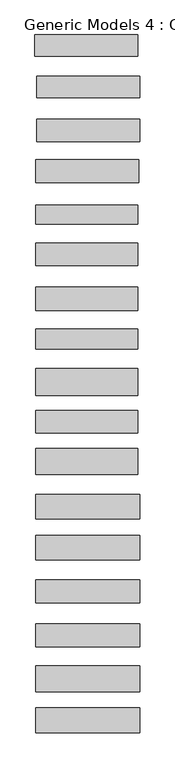
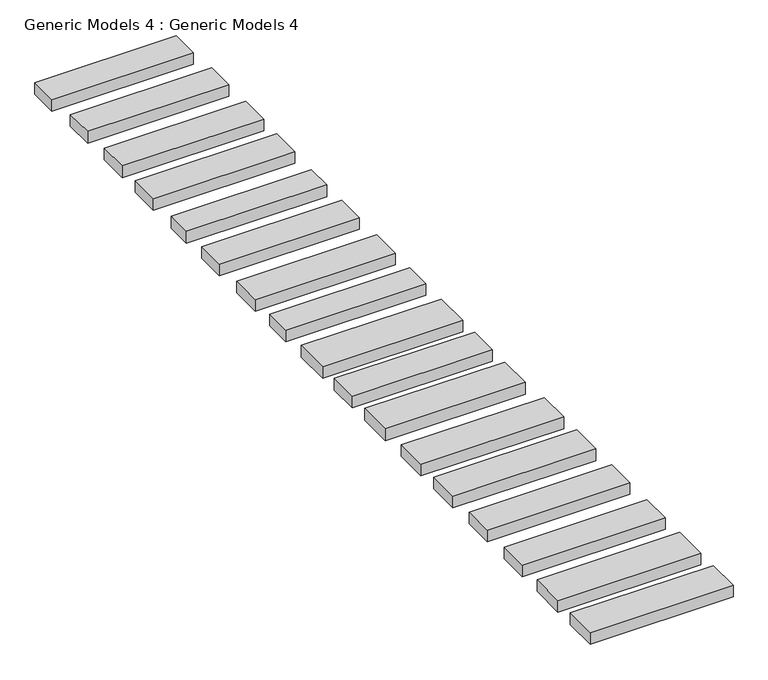
"""IFC4 building model written with IfcOpenShell, lengths in millimetres: proxy geometry, Generic Models 4 : Generic Models 4."""

from ifc_helpers import new_model, si_unit, frame, origin, place, context, project, spatial, polyline, outline, extrude, source, transform, mapped, element, save


def generic_models_4_generic_models_4_6f48c335(model_context):
    return source(origin(), model_context, "Body", "SweptSolid", [
        extrude(outline(polyline([(-33990.9791975, 27174.9938465), (-33990.9791975, 27102.9548339), (-34336.8215134, 27102.9548339), (-34336.8215134, 27174.9938465), (-33990.9791975, 27174.9938465)])), frame((0.0, 0.0, 449.9570313), z_axis=(0.0, 0.0, 1.0), x_axis=(1.0, 0.0, 0.0)), (0.0, 0.0, 1.0), 30.0632812),
        extrude(outline(polyline([(-33984.6291975, 27035.2938465), (-33984.6291975, 26963.2548339), (-34330.4715134, 26963.2548339), (-34330.4715134, 27035.2938465), (-33984.6291975, 27035.2938465)])), frame((0.0, 0.0, 449.9570313), z_axis=(0.0, 0.0, 1.0), x_axis=(1.0, 0.0, 0.0)), (0.0, 0.0, 1.0), 30.0632812),
        extrude(outline(polyline([(-33984.6291975, 26891.4711637), (-33984.6291975, 26815.9588418), (-34330.4715134, 26815.9588418), (-34330.4715134, 26891.4711637), (-33984.6291975, 26891.4711637)])), frame((0.0, 0.0, 449.9570313), z_axis=(0.0, 0.0, 1.0), x_axis=(1.0, 0.0, 0.0)), (0.0, 0.0, 1.0), 30.0632812),
        extrude(outline(polyline([(-33987.8041975, 26754.691992), (-33987.8041975, 26678.491992), (-34333.6465134, 26678.491992), (-34333.6465134, 26754.691992), (-33987.8041975, 26754.691992)])), frame((0.0, 0.0, 449.9570313), z_axis=(0.0, 0.0, 1.0), x_axis=(1.0, 0.0, 0.0)), (0.0, 0.0, 1.0), 30.0632812),
        extrude(outline(polyline([(-34333.6465134, 26602.9245297), (-33990.9791975, 26602.9245297), (-33990.9791975, 26539.0524471), (-34333.6465134, 26539.0524471), (-34333.6465134, 26602.9245297)])), frame((0.0, 0.0, 449.9570313), z_axis=(0.0, 0.0, 1.0), x_axis=(1.0, 0.0, 0.0)), (0.0, 0.0, 1.0), 30.0632812),
        extrude(outline(polyline([(-33990.9791975, 26474.064355), (-33990.9791975, 26399.8367417), (-34333.6465134, 26399.8367417), (-34333.6465134, 26474.064355), (-33990.9791975, 26474.064355)])), frame((0.0, 0.0, 449.9570313), z_axis=(0.0, 0.0, 1.0), x_axis=(1.0, 0.0, 0.0)), (0.0, 0.0, 1.0), 30.0632812),
        extrude(outline(polyline([(-33990.9791975, 26326.1282027), (-33990.9791975, 26248.26707), (-34333.6465134, 26248.26707), (-34333.6465134, 26326.1282027), (-33990.9791975, 26326.1282027)])), frame((0.0, 0.0, 449.9570313), z_axis=(0.0, 0.0, 1.0), x_axis=(1.0, 0.0, 0.0)), (0.0, 0.0, 1.0), 30.0632812),
        extrude(outline(polyline([(-33990.9791975, 26186.497238), (-33990.9791975, 26118.4985154), (-34333.6465134, 26118.4985154), (-34333.6465134, 26186.497238), (-33990.9791975, 26186.497238)])), frame((0.0, 0.0, 449.9570313), z_axis=(0.0, 0.0, 1.0), x_axis=(1.0, 0.0, 0.0)), (0.0, 0.0, 1.0), 30.0632812),
        extrude(outline(polyline([(-33990.9791975, 26052.5760897), (-33990.9791975, 25962.2571757), (-34333.6465134, 25962.2571757), (-34333.6465134, 26052.5760897), (-33990.9791975, 26052.5760897)])), frame((0.0, 0.0, 449.9570313), z_axis=(0.0, 0.0, 1.0), x_axis=(1.0, 0.0, 0.0)), (0.0, 0.0, 1.0), 30.0632812),
        extrude(outline(polyline([(-33990.9791975, 25911.9069765), (-33990.9791975, 25836.1221406), (-34333.6465134, 25836.1221406), (-34333.6465134, 25911.9069765), (-33990.9791975, 25911.9069765)])), frame((0.0, 0.0, 449.9570313), z_axis=(0.0, 0.0, 1.0), x_axis=(1.0, 0.0, 0.0)), (0.0, 0.0, 1.0), 30.0632812),
        extrude(outline(polyline([(-33990.9791975, 25784.2147188), (-33990.9791975, 25697.0102501), (-34333.6465134, 25697.0102501), (-34333.6465134, 25784.2147188), (-33990.9791975, 25784.2147188)])), frame((0.0, 0.0, 449.9570313), z_axis=(0.0, 0.0, 1.0), x_axis=(1.0, 0.0, 0.0)), (0.0, 0.0, 1.0), 30.0632812),
        extrude(outline(polyline([(-33984.3965134, 25629.0115275), (-33984.3965134, 25546.4615275), (-34333.6465134, 25546.4615275), (-34333.6465134, 25629.0115275), (-33984.3965134, 25629.0115275)])), frame((0.0, 0.0, 449.9570313), z_axis=(0.0, 0.0, 1.0), x_axis=(1.0, 0.0, 0.0)), (0.0, 0.0, 1.0), 30.0632812),
        extrude(outline(polyline([(-33984.3965134, 25491.4568596), (-33984.3965134, 25409.9622073), (-34333.6465134, 25409.9622073), (-34333.6465134, 25491.4568596), (-33984.3965134, 25491.4568596)])), frame((0.0, 0.0, 449.9570313), z_axis=(0.0, 0.0, 1.0), x_axis=(1.0, 0.0, 0.0)), (0.0, 0.0, 1.0), 30.0632812),
        extrude(outline(polyline([(-33984.3965134, 25341.9634847), (-33984.3965134, 25265.6595746), (-34333.6465134, 25265.6595746), (-34333.6465134, 25341.9634847), (-33984.3965134, 25341.9634847)])), frame((0.0, 0.0, 449.9570313), z_axis=(0.0, 0.0, 1.0), x_axis=(1.0, 0.0, 0.0)), (0.0, 0.0, 1.0), 30.0632812),
        extrude(outline(polyline([(-33984.3965134, 25193.5082583), (-33984.3965134, 25116.1661998), (-34333.6465134, 25116.1661998), (-34333.6465134, 25193.5082583), (-33984.3965134, 25193.5082583)])), frame((0.0, 0.0, 449.9570313), z_axis=(0.0, 0.0, 1.0), x_axis=(1.0, 0.0, 0.0)), (0.0, 0.0, 1.0), 30.0632812),
        extrude(outline(polyline([(-33984.3965134, 25053.8772936), (-33984.3965134, 24965.1156022), (-34333.6465134, 24965.1156022), (-34333.6465134, 25053.8772936), (-33984.3965134, 25053.8772936)])), frame((0.0, 0.0, 449.9570313), z_axis=(0.0, 0.0, 1.0), x_axis=(1.0, 0.0, 0.0)), (0.0, 0.0, 1.0), 30.0632812),
        extrude(outline(polyline([(-33984.3965134, 24912.4408533), (-33984.3965134, 24828.4862406), (-34333.6465134, 24828.4862406), (-34333.6465134, 24912.4408533), (-33984.3965134, 24912.4408533)])), frame((0.0, 0.0, 449.9570313), z_axis=(0.0, 0.0, 1.0), x_axis=(1.0, 0.0, 0.0)), (0.0, 0.0, 1.0), 30.0632812),
    ])


if __name__ == "__main__":
    model = new_model("IFC4")
    model_context = context("Model", 3, world=origin())
    ifc_project = project(units=[si_unit("LENGTHUNIT", "METRE", prefix="MILLI")], contexts=[model_context])
    site = spatial("IfcSite", under=ifc_project)
    building = spatial("IfcBuilding", under=site)
    placement = place(None, origin())
    generic_models_4_generic_models_4_shape = generic_models_4_generic_models_4_6f48c335(model_context)
    element("IfcBuildingElementProxy", 1, Name="Generic Models 4 : Generic Models 4", ObjectType="Generic Models 4 : Generic Models 4", at=placement, inside=building, context=model_context, shape_type="MappedRepresentation", body=[
        mapped(generic_models_4_generic_models_4_shape, transform((0.0, 0.0, 0.0), x_axis=(1.0, 0.0, 0.0), y_axis=(0.0, 1.0, 0.0), z_axis=(0.0, 0.0, 1.0))),
    ])
    save(model, "model.ifc")
